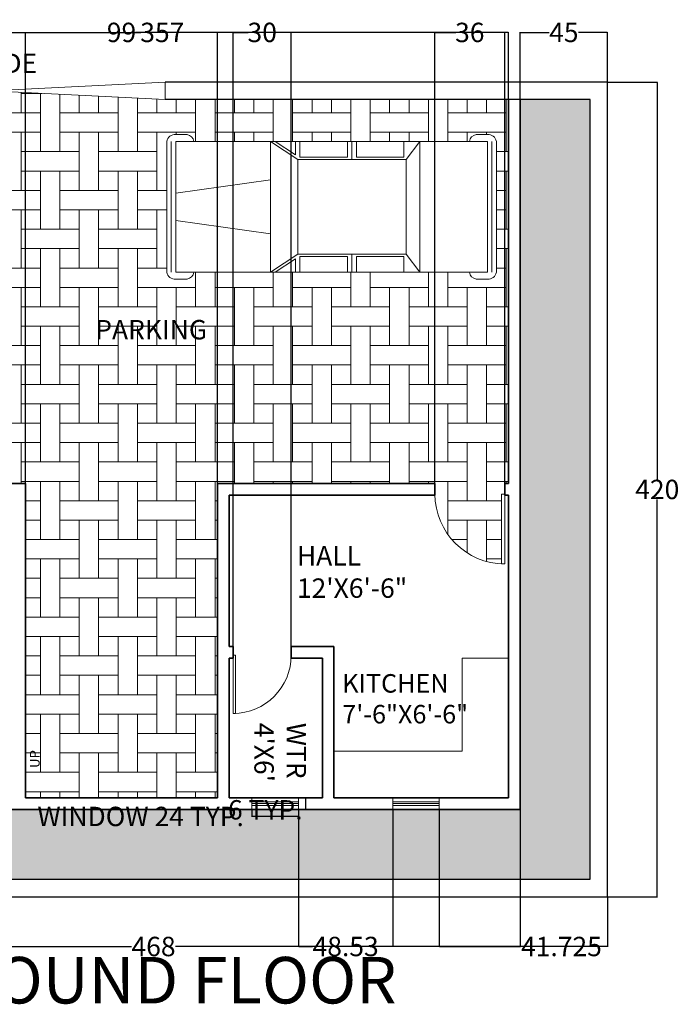
# Model space of a CAD drawing. Units: inches. Extents: x 377 to 1481, y 110 to 618.
# Tile 1 of 3: x 579 to 919, y 110 to 618. Entities that reach past the tile are written whole.
import ezdxf

# ---------------------------------------------------------------- set-up
doc = ezdxf.new("R2010")
doc.units = ezdxf.units.IN
doc.header["$MEASUREMENT"] = 0
for name, color, linetype, lineweight in [('A-ANNO-DIMS', 2, 'Continuous', 18), ('A-ANNO-TEXT', 7, 'Continuous', 18), ('A-ANNO-TITL', 7, 'Continuous', 35), ('A-AREA-IDEN', 7, 'Continuous', 18), ('A-DOOR', 4, 'Continuous', 18), ('A-EQPM-VEHI', 8, 'Continuous', 13), ('A-FLOR-FIXT', 8, 'Continuous', 20), ('A-GLAZ', 4, 'Continuous', 18), ('A-WALL', 7, 'Continuous', 35), ('C-PROP', 7, 'Continuous', 25), ('L-SITE-GATE', 3, 'Continuous', 18)]:
    doc.layers.add(name, color=color, linetype=linetype, lineweight=lineweight)
doc.layers.add('A-FLOR-PATT', color=252, linetype='Continuous', lineweight=13, true_color=0x939598)
doc.layers.add('L-PLNT-PATT', color=85, linetype='Continuous', lineweight=13, true_color=0x58ba48)
doc.styles.get("Standard").update_dxf_attribs({"font": 'arial.ttf'})
doc.dimstyles.get("Standard").update_dxf_attribs({"dimtxt": 10, "dimasz": 0.18, "dimexe": 0.18, "dimexo": 0.0625, "dimgap": 0.09, "dimtad": 0, "dimtih": 1, "dimtoh": 1, "dimdec": 0, "dimzin": 0, "dimdsep": 46, "dimlunit": 3, "dimtxsty": 'Standard', "dimcen": 0.09, "dimadec": 0, "dimazin": 0, "dimtfac": 1, "dimtdec": 0, "dimtofl": 0, "dimtmove": 0, "dimatfit": 3, "dimfxl": 1, "dimtolj": 1, "dimtzin": 0, "dimarcsym": 0})

# ---------------------------------------------------------------- blocks, each defined once
blk = doc.blocks.new('*U9')
for p, q in [((0, 0), (0, -5.999999999999999)), ((40, -6e-16), (40, -6))]:
    blk.add_line(p, q)
blk.add_lwpolyline([(0, 0), (7.1e-15, 40), (1.750000000000007, 40), (1.75, -7e-16)], close=True)
blk.add_arc((0, 0), 40, 7e-15, 90)
blk = doc.blocks.new('*U3')
for p, q in [((0, 0), (0, -5.999999999999999)), ((-40, -6e-16), (-40, -6))]:
    blk.add_line(p, q)
blk.add_lwpolyline([(0, 0), (-7.1e-15, 40), (-1.750000000000007, 40), (-1.75, -7e-16)], close=True)
blk.add_arc((0, 0), 40, 90, 180)
blk = doc.blocks.new('*U12')
for p, q in [((5.442702667415691, 42.31050314550827), (12.1182799520597, 42.31050314550827)), ((189.6886357235905, 42.31050314550827), (183.0130584389465, 42.31050314550827)), ((0.1022408397004799, -0.4060708604432933), (0.1022408397004799, 38.34966062328632)), ((2.772471753558085, -0.4131914762133988), (2.772471753558085, 38.30515677472187)), ((5.442702667415691, -0.4060708604432933), (5.442702667415691, 38.24285138673173)), ((5.446262975300346, 38.30515677472187), (16.12362632284611, 38.30515677472187)), ((16.12362632284611, 38.30515677472187), (180.3428275250889, 38.30515677472187)), ((61.5175518584254, -0.4131914762133988), (61.5175518584254, 38.30515677472187)), ((61.5175518584254, 38.30515677472187), (77.53893734157104, 27.62423311929143)), ((64.18778277228301, 38.30515677472187), (76.20382188464222, 30.29446403314904)), ((76.20382188464222, 30.29446403314904), (76.20382188464222, 38.30515677472187)), ((78.87405279849985, 38.30515677472187), (78.87405279849985, 28.95934857622023)), ((106.9114773940047, 28.95934857622023), (106.9114773940047, 38.30515677472187)), ((109.5817083078623, 27.62423311929143), (109.5817083078623, 38.30515677472187)), ((112.2519392217199, 38.30515677472187), (112.2519392217199, 28.95934857622023)), ((140.2893638172247, 28.95934857622023), (140.2893638172247, 38.30515677472187)), ((141.6244792741536, 27.62423311929143), (149.6351720157264, 38.30515677472187)), ((149.6351720157264, -0.4131914762133988), (149.6351720157264, 38.30515677472187)), ((189.685075415705, 38.30515677472187), (179.00771206816, 38.30515677472187)), ((189.6886357235905, -0.4060708604432933), (189.6886357235905, 38.24285138673173)), ((192.3588666374481, -0.4131914762133988), (192.3588666374481, 38.30515677472187)), ((195.0290975513057, -0.4060708604432933), (195.0290975513057, 38.34966062328632)), ((77.53893734157104, 27.62423311929143), (141.6244792741536, 27.62423311929143)), ((77.53893734157104, -0.4131914762133988), (77.53893734157104, 27.62423311929143)), ((78.87405279849985, 28.95934857622023), (106.9114773940047, 28.95934857622023)), ((112.2519392217199, 28.95934857622023), (140.2893638172247, 28.95934857622023)), ((141.6244792741536, -0.4131914762133988), (141.6244792741536, 27.62423311929143)), ((5.442702667415691, 7.597501265359397), (61.5175518584254, 15.60819400693222)), ((0.1022408397004799, -0.4203120919839308), (0.1022408397004799, -39.17604357571315)), ((2.772471753558085, -0.4131914762133988), (2.772471753558085, -39.13153972714869)), ((5.442702667415691, -0.4203120919839308), (5.442702667415691, -39.06923433915853)), ((61.5175518584254, -0.4131914762133988), (61.5175518584254, -39.13153972714869)), ((77.53893734157104, -0.4131914762133988), (77.53893734157104, -28.45061607171829)), ((141.6244792741536, -0.4131914762133988), (141.6244792741536, -28.45061607171829)), ((149.6351720157264, -0.4131914762133988), (149.6351720157264, -39.13153972714869)), ((189.6886357235905, -0.4203120919839308), (189.6886357235905, -39.06923433915853)), ((192.3588666374481, -0.4131914762133988), (192.3588666374481, -39.13153972714869)), ((195.0290975513057, -0.4203120919839308), (195.0290975513057, -39.17604357571315)), ((5.442702667415691, -8.423884217786224), (61.5175518584254, -16.43457695935905)), ((61.5175518584254, -39.13153972714869), (77.53893734157104, -28.45061607171829)), ((77.53893734157104, -28.45061607171829), (141.6244792741536, -28.45061607171829)), ((109.5817083078623, -28.45061607171829), (109.5817083078623, -39.13153972714869)), ((141.6244792741536, -28.45061607171829), (149.6351720157264, -39.13153972714869)), ((64.18778277228301, -39.13153972714869), (76.20382188464222, -31.12084698557587)), ((76.20382188464222, -31.12084698557587), (76.20382188464222, -39.13153972714869)), ((78.87405279849985, -39.13153972714869), (78.87405279849985, -29.78573152864706)), ((78.87405279849985, -29.78573152864706), (106.9114773940047, -29.78573152864706)), ((106.9114773940047, -29.78573152864706), (106.9114773940047, -39.13153972714869)), ((112.2519392217199, -29.78573152864706), (140.2893638172247, -29.78573152864706)), ((112.2519392217199, -39.13153972714869), (112.2519392217199, -29.78573152864706)), ((140.2893638172247, -29.78573152864706), (140.2893638172247, -39.13153972714869)), ((5.446262975300346, -39.13153972714869), (16.12362632284611, -39.13153972714869)), ((16.12362632284611, -39.13153972714869), (180.3428275250889, -39.13153972714869)), ((189.685075415705, -39.13153972714869), (179.00771206816, -39.13153972714869)), ((5.442702667415691, -43.1368860979351), (12.1182799520597, -43.1368860979351)), ((189.6886357235905, -43.1368860979351), (183.0130584389465, -43.1368860979351))]:
    blk.add_line(p, q)
for centre, radius, start, end in [((5.058189415819978, 37.26020641043229), 5.064858394326255, 85.64553999999978, 168.0943000000001), ((11.4507222235953, 37.63759904625749), 4.720341641512461, 8.130111000000149, 81.8699600000003), ((183.6806161674108, 37.63759904625749), 4.720341641512461, 98.1300399999997, 171.8698999999996), ((190.0731489751854, 37.26020641043229), 5.064858394326255, 11.90573999999997, 94.35446000000022), ((5.058189415819978, -38.08658936285912), 5.064858394326255, 191.9056999999999, 274.3545000000004), ((11.4507222235953, -38.46398199868429), 4.720341641512461, 278.1300000000006, 351.8698999999996), ((183.6806161674108, -38.46398199868429), 4.720341641512461, 188.1301000000004, 261.8699999999993), ((190.0731489751854, -38.08658936285912), 5.064858394326255, 265.6454999999995, 348.0943000000001)]:
    blk.add_arc(centre, radius, start, end)
blk = doc.blocks.new('WIN-24IN')
for p, q in [((8.90267408522e-05, 6.000397743999627), (8.90267408522e-05, 0.0003977439995708)), ((24.00008902674085, 6.000397743999627), (24.00008902674085, 0.0003977439995708)), ((24.00008902674085, 4.000397743999599), (8.90267408522e-05, 4.000397743999599)), ((24.00008902674085, 3.000397743999599), (8.90267408522e-05, 3.000397743999599)), ((24.00008902674085, 2.000397743999599), (8.90267408522e-05, 2.000397743999599))]:
    blk.add_line(p, q)
blk = doc.blocks.new('*D17')
at = {"layer": 'A-ANNO-DIMS', "color": 0, "lineweight": -2, "transparency": 16777216}
for p, q in [((699.0626046596035, 210.7768977439996), (699.0626046596035, 207.0593977439996)), ((723.0626046596035, 210.7768977439996), (723.0626046596035, 207.0593977439996)), ((699.0626046596035, 207.2393977439996), (698.8826046596034, 207.2393977439996)), ((722.8826046596035, 207.2393977439996), (699.2426046596034, 207.2393977439996))]:
    blk.add_line(p, q, dxfattribs=at)
at = {"layer": 'A-ANNO-DIMS', "color": 0, "lineweight": 100, "transparency": 16777216}
for points in [[(699.2426046596034, 207.2693977439996), (699.2426046596034, 207.2093977439996), (699.0626046596035, 207.2393977439996)], [(722.8826046596035, 207.2693977439996), (722.8826046596035, 207.2093977439996), (723.0626046596035, 207.2393977439996)]]:
    blk.add_solid(points, dxfattribs=at)
at = {"layer": 'Defpoints', "color": 0, "lineweight": 100, "transparency": 16777216}
for p in [(699.0626046596035, 210.8393977439996), (723.0626046596035, 210.8393977439996), (699.0626046596035, 207.2393977439996)]:
    blk.add_point(p, dxfattribs=at)
at = {"layer": 'A-ANNO-DIMS', "color": 0, "transparency": 16777216, "insert": (641.6609539092624, 207.2393977439996), "char_height": 10, "attachment_point": 5}
blk.add_mtext('\\A1;WINDOW 24 TYP.', dxfattribs=at)
blk = doc.blocks.new('*D18')
at = {"layer": 'A-ANNO-DIMS', "color": 0, "lineweight": -2, "transparency": 16777216}
for p, q in [((723.1251046596037, 216.8393977439997), (726.8426046596039, 216.8393977439997)), ((726.6626046596039, 216.6593977439998), (726.6626046596039, 211.0193977439997)), ((723.1251046596037, 210.8393977439997), (726.8426046596039, 210.8393977439997)), ((726.6626046596039, 210.6593977439997), (726.482604659604, 210.6593977439997)), ((726.6626046596039, 210.8393977439997), (726.6626046596039, 210.6593977439997))]:
    blk.add_line(p, q, dxfattribs=at)
at = {"layer": 'A-ANNO-DIMS', "color": 0, "lineweight": 100, "transparency": 16777216}
for points in [[(726.632604659604, 216.6593977439998), (726.692604659604, 216.6593977439998), (726.6626046596039, 216.8393977439997)], [(726.632604659604, 211.0193977439997), (726.692604659604, 211.0193977439997), (726.6626046596039, 210.8393977439997)]]:
    blk.add_solid(points, dxfattribs=at)
at = {"layer": 'Defpoints', "color": 0, "lineweight": 100, "transparency": 16777216}
for p in [(723.0626046596037, 216.8393977439997), (723.0626046596037, 210.8393977439997), (726.6626046596039, 210.8393977439997)]:
    blk.add_point(p, dxfattribs=at)
at = {"layer": 'A-ANNO-DIMS', "color": 0, "transparency": 16777216, "insert": (705.9117042503268, 210.6593977439994), "char_height": 10, "attachment_point": 5}
blk.add_mtext('\\A1;6 TYP.', dxfattribs=at)
blk = doc.blocks.new('*D27')
at = {"layer": 'A-ANNO-DIMS', "color": 0, "lineweight": -2, "transparency": 16777216}
for p, q in [((414.320847, 165.776898), (414.320847, 140.009398)), ((882.3208469999998, 165.776898), (882.3208469999998, 140.009398)), ((414.500847, 140.189398), (636.9723203969986, 140.189398)), ((882.1408469999999, 140.189398), (659.6693736030013, 140.189398))]:
    blk.add_line(p, q, dxfattribs=at)
at = {"layer": 'A-ANNO-DIMS', "color": 0, "lineweight": 100, "transparency": 16777216}
for points in [[(414.500847, 140.219398), (414.500847, 140.159398), (414.320847, 140.189398)], [(882.1408469999999, 140.219398), (882.1408469999999, 140.159398), (882.3208469999998, 140.189398)]]:
    blk.add_solid(points, dxfattribs=at)
at = {"layer": 'Defpoints', "color": 0, "lineweight": 100, "transparency": 16777216}
for p in [(414.320847, 165.839398), (882.3208469999998, 165.839398), (882.3208469999998, 140.189398)]:
    blk.add_point(p, dxfattribs=at)
at = {"layer": 'A-ANNO-DIMS', "color": 0, "transparency": 16777216, "insert": (648.320847, 140.189398), "char_height": 10, "attachment_point": 5}
blk.add_mtext('\\A1;468', dxfattribs=at)
blk = doc.blocks.new('*D28')
at = {"layer": 'A-ANNO-DIMS', "color": 0, "lineweight": -2, "transparency": 16777216}
for p, q in [((882.3833470000003, 585.8393980000001), (908.1508470000009, 585.8393980000001)), ((907.970847000001, 585.6593980000002), (907.970847000001, 381.035127877217)), ((907.970847000001, 166.019398), (907.970847000001, 370.6436681227832)), ((882.3833470000003, 165.839398), (908.1508470000009, 165.839398))]:
    blk.add_line(p, q, dxfattribs=at)
at = {"layer": 'A-ANNO-DIMS', "color": 0, "lineweight": 100, "transparency": 16777216}
for points in [[(907.9408470000009, 585.6593980000002), (908.0008470000009, 585.6593980000002), (907.970847000001, 585.8393980000001)], [(907.9408470000011, 166.019398), (908.0008470000009, 166.019398), (907.970847000001, 165.839398)]]:
    blk.add_solid(points, dxfattribs=at)
at = {"layer": 'Defpoints', "color": 0, "lineweight": 100, "transparency": 16777216}
for p in [(882.3208470000004, 585.8393980000001), (907.970847000001, 585.8393980000001), (882.3208470000004, 165.839398)]:
    blk.add_point(p, dxfattribs=at)
at = {"layer": 'A-ANNO-DIMS', "color": 0, "transparency": 16777216, "insert": (907.9708470000008, 375.8393979999998), "char_height": 10, "attachment_point": 5}
blk.add_mtext('\\A1;420', dxfattribs=at)
blk = doc.blocks.new('*D30')
at = {"layer": 'A-ANNO-DIMS', "color": 0, "lineweight": -2, "transparency": 16777216}
for p, q in [((474.31833, 576.9018979999998), (474.31833, 611.6693979999999)), ((474.49833, 611.489398), (641.6859322926329, 611.489398)), ((831.1408469999999, 611.489398), (663.953244707367, 611.489398)), ((831.3208469999998, 576.9018979999998), (831.3208469999998, 611.6693979999999))]:
    blk.add_line(p, q, dxfattribs=at)
at = {"layer": 'A-ANNO-DIMS', "color": 0, "lineweight": 100, "transparency": 16777216}
for points in [[(474.49833, 611.519398), (474.49833, 611.4593980000001), (474.31833, 611.489398)], [(831.1408469999999, 611.519398), (831.1408469999999, 611.4593980000001), (831.3208469999998, 611.489398)]]:
    blk.add_solid(points, dxfattribs=at)
at = {"layer": 'Defpoints', "color": 0, "lineweight": 100, "transparency": 16777216}
for p in [(831.3208469999998, 611.489398), (474.31833, 576.8393979999998), (831.3208469999998, 576.8393979999998)]:
    blk.add_point(p, dxfattribs=at)
at = {"layer": 'A-ANNO-DIMS', "color": 0, "transparency": 16777216, "insert": (652.8195885, 611.489398), "char_height": 10, "attachment_point": 5}
blk.add_mtext('\\A1;357', dxfattribs=at)
blk = doc.blocks.new('*D31')
at = {"layer": 'A-ANNO-DIMS', "color": 0, "lineweight": -2, "transparency": 16777216}
for p, q in [((837.3208469999998, 576.9018979999998), (837.3208469999998, 611.6693979999999)), ((837.5008469999999, 611.489398), (852.3297555948158, 611.489398)), ((882.1408469999999, 611.489398), (867.3119384051842, 611.489398)), ((882.3208469999998, 585.901898), (882.3208469999998, 611.6693979999999))]:
    blk.add_line(p, q, dxfattribs=at)
at = {"layer": 'A-ANNO-DIMS', "color": 0, "lineweight": 100, "transparency": 16777216}
for points in [[(837.5008469999999, 611.519398), (837.5008469999999, 611.4593980000001), (837.3208469999998, 611.489398)], [(882.1408469999999, 611.519398), (882.1408469999999, 611.4593980000001), (882.3208469999998, 611.489398)]]:
    blk.add_solid(points, dxfattribs=at)
at = {"layer": 'Defpoints', "color": 0, "lineweight": 100, "transparency": 16777216}
for p in [(882.3208469999998, 611.489398), (882.3208469999998, 585.8393979999998), (837.3208469999998, 576.8393979999998)]:
    blk.add_point(p, dxfattribs=at)
at = {"layer": 'A-ANNO-DIMS', "color": 0, "transparency": 16777216, "insert": (859.8208469999998, 611.489398), "char_height": 10, "attachment_point": 5}
blk.add_mtext('\\A1;45', dxfattribs=at)
blk = doc.blocks.new('*D35')
at = {"layer": 'A-ANNO-DIMS', "color": 0, "lineweight": -2, "transparency": 16777216}
for p, q in [((582.31833, 216.901898), (582.31833, 611.669398)), ((582.4983299999998, 611.489398), (624.5570100552522, 611.489398)), ((681.1408469999999, 611.489398), (639.0821669447477, 611.489398)), ((681.3208469999998, 216.901898), (681.3208469999998, 611.669398))]:
    blk.add_line(p, q, dxfattribs=at)
at = {"layer": 'A-ANNO-DIMS', "color": 0, "lineweight": 100, "transparency": 16777216}
for points in [[(582.4983299999998, 611.519398), (582.4983299999998, 611.4593980000001), (582.31833, 611.489398)], [(681.1408469999999, 611.519398), (681.1408469999999, 611.4593980000001), (681.3208469999998, 611.489398)]]:
    blk.add_solid(points, dxfattribs=at)
at = {"layer": 'Defpoints', "color": 0, "lineweight": 100, "transparency": 16777216}
for p in [(681.3208469999998, 611.489398), (582.31833, 216.839398), (681.3208469999998, 216.839398)]:
    blk.add_point(p, dxfattribs=at)
at = {"layer": 'A-ANNO-DIMS', "color": 0, "transparency": 16777216, "insert": (631.8195885, 611.489398), "char_height": 10, "attachment_point": 5}
blk.add_mtext('\\A1;99', dxfattribs=at)
blk = doc.blocks.new('*D36')
at = {"layer": 'A-ANNO-DIMS', "color": 0, "lineweight": -2, "transparency": 16777216}
for p, q in [((793.3208469999998, 378.901898), (793.3208469999998, 611.6693979999999)), ((793.5008469999999, 611.489398), (804.075321761255, 611.489398)), ((829.140847, 611.489398), (818.5663722387449, 611.489398)), ((829.3208469999998, 378.901898), (829.3208469999998, 611.6693979999999))]:
    blk.add_line(p, q, dxfattribs=at)
at = {"layer": 'A-ANNO-DIMS', "color": 0, "lineweight": 100, "transparency": 16777216}
for points in [[(793.5008469999999, 611.519398), (793.5008469999999, 611.4593980000001), (793.3208469999998, 611.489398)], [(829.140847, 611.519398), (829.140847, 611.4593980000001), (829.3208469999998, 611.489398)]]:
    blk.add_solid(points, dxfattribs=at)
at = {"layer": 'Defpoints', "color": 0, "lineweight": 100, "transparency": 16777216}
for p in [(829.3208469999998, 611.489398), (793.3208469999998, 378.839398), (829.3208469999998, 378.839398)]:
    blk.add_point(p, dxfattribs=at)
at = {"layer": 'A-ANNO-DIMS', "color": 0, "transparency": 16777216, "insert": (811.320847, 611.489398), "char_height": 10, "attachment_point": 5}
blk.add_mtext('\\A1;36', dxfattribs=at)
blk = doc.blocks.new('*D37')
at = {"layer": 'A-ANNO-DIMS', "color": 0, "lineweight": -2, "transparency": 16777216}
for p, q in [((689.3208469999998, 294.901898), (689.3208469999998, 611.6693979999999)), ((689.5008469999999, 611.489398), (697.0889643260573, 611.489398)), ((719.1408469999999, 611.489398), (711.5527296739426, 611.489398)), ((719.320847, 294.901898), (719.320847, 611.6693979999999))]:
    blk.add_line(p, q, dxfattribs=at)
at = {"layer": 'A-ANNO-DIMS', "color": 0, "lineweight": 100, "transparency": 16777216}
for points in [[(689.5008469999999, 611.519398), (689.5008469999999, 611.4593980000001), (689.3208469999998, 611.489398)], [(719.1408469999999, 611.519398), (719.1408469999999, 611.4593980000001), (719.320847, 611.489398)]]:
    blk.add_solid(points, dxfattribs=at)
at = {"layer": 'Defpoints', "color": 0, "lineweight": 100, "transparency": 16777216}
for p in [(719.320847, 611.489398), (689.3208469999998, 294.839398), (719.320847, 294.839398)]:
    blk.add_point(p, dxfattribs=at)
at = {"layer": 'A-ANNO-DIMS', "color": 0, "transparency": 16777216, "insert": (704.3208469999998, 611.489398), "char_height": 10, "attachment_point": 5}
blk.add_mtext('\\A1;30', dxfattribs=at)
blk = doc.blocks.new('*D38')
at = {"layer": 'A-ANNO-DIMS', "color": 0, "lineweight": -2, "transparency": 16777216}
for p, q in [((723.0626049999998, 210.776898), (723.0626049999998, 140.009398)), ((771.596188, 210.776898), (771.596188, 140.009398)), ((723.2426049999999, 140.189398), (730.1657266500682, 140.189398)), ((771.416188, 140.189398), (764.4930663499318, 140.189398))]:
    blk.add_line(p, q, dxfattribs=at)
at = {"layer": 'A-ANNO-DIMS', "color": 0, "lineweight": 100, "transparency": 16777216}
for points in [[(723.2426049999999, 140.219398), (723.2426049999999, 140.159398), (723.0626049999998, 140.189398)], [(771.416188, 140.219398), (771.416188, 140.159398), (771.596188, 140.189398)]]:
    blk.add_solid(points, dxfattribs=at)
at = {"layer": 'Defpoints', "color": 0, "lineweight": 100, "transparency": 16777216}
for p in [(723.0626049999998, 210.839398), (771.596188, 210.839398), (771.596188, 140.189398)]:
    blk.add_point(p, dxfattribs=at)
at = {"layer": 'A-ANNO-DIMS', "color": 0, "transparency": 16777216, "insert": (747.3293965, 140.189398), "char_height": 10, "attachment_point": 5}
blk.add_mtext('\\A1;48.53', dxfattribs=at)
blk = doc.blocks.new('*D39')
at = {"layer": 'A-ANNO-DIMS', "color": 0, "lineweight": -2, "transparency": 16777216}
for p, q in [((795.596188, 210.776898), (795.596188, 140.009398)), ((837.3208469999998, 210.776898), (837.3208469999998, 140.009398)), ((795.7761879999999, 140.189398), (837.140847, 140.189398)), ((837.3208469999998, 140.189398), (837.500847, 140.189398))]:
    blk.add_line(p, q, dxfattribs=at)
at = {"layer": 'A-ANNO-DIMS', "color": 0, "lineweight": 100, "transparency": 16777216}
for points in [[(795.7761879999999, 140.219398), (795.7761879999999, 140.159398), (795.596188, 140.189398)], [(837.140847, 140.219398), (837.140847, 140.159398), (837.3208469999998, 140.189398)]]:
    blk.add_solid(points, dxfattribs=at)
at = {"layer": 'Defpoints', "color": 0, "lineweight": 100, "transparency": 16777216}
for p in [(795.596188, 210.839398), (837.3208469999998, 210.839398), (837.3208469999998, 140.189398)]:
    blk.add_point(p, dxfattribs=at)
at = {"layer": 'A-ANNO-DIMS', "color": 0, "transparency": 16777216, "insert": (858.5867542305592, 140.189398), "char_height": 10, "attachment_point": 5}
blk.add_mtext('\\A1;41.725', dxfattribs=at)

msp = doc.modelspace()

# ---------------------------------------------------------------- hatches: boundary and pattern name
at = {"layer": 'A-FLOR-PATT'}
h = msp.add_hatch(dxfattribs=at)
h.set_pattern_fill('±ÀÖ¯²ÄÁÏ', color=256, scale=20)
h.set_pattern_definition([(0, (0, 0), (20, 20), [30, -10]), (0, (0, 10), (20, 20), [30, -10]), (90, (10, 10), (-20, 20), [30, -10]), (90, (20, 10), (-20, 20), [30, -10])])
h.paths.add_polyline_path([(831.3208470620848, 576.8393977439996), (654.3183302215624, 576.8393977439996), (564.3183302215629, 581.3393977439996), (474.3183302215626, 576.8393977439996), (474.3183302215626, 378.8393977439996), (582.3183302215626, 378.8393977439995), (582.3183302215626, 216.8393977439996), (681.320847062085, 216.8393977439997), (681.3208470620849, 378.8393977439995), (793.3762999136519, 378.8393977439995), (793.3762999136519, 373.4477156717346, 0.4014527144963569), (827.7482731243409, 337.537585054926), (827.7482731243409, 373.4477156717346), (829.3208470620848, 373.4477156717346), (829.3208470620848, 378.8393977439996), (831.3208470620848, 378.8393977439995)])
h.paths.add_polyline_path([(655.1112320992189, 487.8017993641329), (655.1112320992189, 521.5563777088427), (655.1112320992189, 555.3233738998766, -0.3760864404517753), (659.767292319398, 558.8161256031975), (665.5887632688018, 558.8161256031975, -0.3333350785240507), (669.0813054040638, 555.3236063246482), (669.0813092134161, 555.3236063246482), (811.1104303504404, 555.3236063246482, -0.3333350785240531), (814.6029724857026, 558.8161256031975), (820.4244434351054, 558.8161256031975, -0.3760864404519927), (825.0805036552854, 555.3233738998733), (825.0805036552854, 521.5687955551666), (825.0805036552854, 487.8017993641362, -0.3760864404520696), (820.4244434351043, 484.3090476608121), (814.6029724857024, 484.3090476608121, -0.3333350785240366), (811.1104303504404, 487.8015669393615), (811.1104265410881, 487.8015669393615), (669.0813054040638, 487.8015669393615, -0.3333350785240358), (665.588763268802, 484.3090476608121), (659.7672923193994, 484.3090476608121, -0.3760864404518541)], flags=16)
h.paths.add_polyline_path([(659.7679244706181, 521.5563777088427), (659.7679244706181, 528.5476251891034), (708.6631943703085, 535.532663746202), (708.6631943703085, 555.3236063246482), (722.6332714845057, 546.01022158185), (778.5135799412946, 546.01022158185), (785.4986184983933, 555.3236063246482), (785.4986184983933, 521.5625866320047), (785.4986184983933, 487.8015669393614), (778.5135799412946, 497.1149516821596), (722.6332714845057, 497.1149516821596), (708.6631943703085, 487.8015669393615), (708.6631943703085, 507.5925095178076), (659.7679244706181, 514.5775480749062)], flags=0)
edge = h.paths.add_edge_path(flags=16)
edge.add_ellipse((512.141418614859, 584.5696558424829), major_axis=(-204.7255748268525, 9.67931e-11), ratio=0.8423038695443797, start_angle=100.2095389971704, end_angle=102.44462729347111, ccw=False)
edge.add_ellipse((565.7338664611478, 273.648778987746), major_axis=(168.2852536317261, 6.42065e-11), ratio=0.842303869543657, start_angle=99.25656600717964, end_angle=102.5549326441154)
edge.add_line((534.707768362197, 412.9662154153117), (530.5983486771285, 410.6938254662535))
edge.add_line((530.5983486771285, 410.6938254662535), (526.4889289920602, 412.9662154153116))
edge.add_ellipse((495.4628308931093, 273.648778987746), major_axis=(168.2852536315943, 6.1815e-11), ratio=0.8423038695442986, start_angle=77.44506735584166, end_angle=80.74343399277738)
edge.add_ellipse((549.0552787394023, 584.5696558424856), major_axis=(204.7255748269201, 3.28788e-11), ratio=0.8423038695441253, start_angle=257.5553727065455, end_angle=259.7904610028463, ccw=False)
edge.add_ellipse((928.8888750783977, 435.9044437085582), major_axis=(-417.9823698359099, 1.184e-13), ratio=0.842303869543927, start_angle=-2.1985405659551134, end_angle=2.8637146078376077, ccw=False)
edge.add_ellipse((526.9857163546047, 500.9000910277084), major_axis=(60.20166025916774, 4.181e-13), ratio=0.8423038695439812, start_angle=252.2800467772492, end_angle=265.917589308849)
edge.add_line((523.3730840320812, 450.283383470902), (537.8236133221772, 450.283383470902))
edge.add_ellipse((534.2109809996527, 500.9000910277083), major_axis=(60.201660259169, 1.2736e-12), ratio=0.8423038695439622, start_angle=-85.91758930885108, end_angle=-72.28004677725126)
edge.add_ellipse((132.3078222758608, 435.9044437085587), major_axis=(-417.9823698359087, 2.3459e-12), ratio=0.8423038695438743, start_angle=177.1362853921626, end_angle=182.1985405659555, ccw=False)
edge = h.paths.add_edge_path(flags=16)
edge.add_ellipse((534.2109809996541, 501.4974298966528), major_axis=(54.83387102201502, 2.4993e-12), ratio=0.8423038695439453, start_angle=-85.7225790369485, end_angle=-68.16504620329431, ccw=False)
edge.add_line((537.6586440135299, 455.4020319851987), (523.5380533407272, 455.4020319851987))
edge.add_ellipse((526.985716354604, 501.4974298966517), major_axis=(-54.8338710220135, 2.0245e-12), ratio=0.8423038695439498, start_angle=68.16504620329238, end_angle=85.72257903694663, ccw=False)
edge.add_line((509.4513084570433, 457.7357275014352), (510.9164148538646, 468.7168197280619))
edge.add_ellipse((528.721139195539, 511.0893217744386), major_axis=(53.3633742937202, 3.469e-13), ratio=0.8423038695439728, start_angle=247.2080851224096, end_angle=265.1299304028639)
edge.add_line((524.9011977337861, 466.2564549519428), (536.295499620471, 466.2564549519428))
edge.add_ellipse((532.4755581587168, 511.0893217744494), major_axis=(53.36337429373605, 3.8424e-12), ratio=0.8423038695439261, start_angle=-85.12993040286842, end_angle=-67.20808512241756)
edge.add_line((550.2802825003928, 468.7168197280617), (551.7453888972141, 457.735727501435))
edge = h.paths.add_edge_path(flags=0)
edge.add_line((542.111699473761, 444.9337137407289), (542.111699473761, 435.0025221262431))
edge.add_line((542.111699473761, 435.0025221262431), (538.2562464159993, 432.3163569622979))
edge.add_line((538.2562464159993, 432.3163569622979), (536.972632243019, 432.3163569622979))
edge.add_line((536.972632243019, 432.3163569622979), (536.972632243019, 430.7404435434111))
edge.add_ellipse((499.3077352576486, 430.740443543411), major_axis=(-37.66489698537048, 7.634e-13), ratio=0.8423038695439682, start_angle=150.5614304020218, end_angle=180.0000000000012, ccw=False)
edge.add_ellipse((561.8889620966085, 430.740443543411), major_axis=(37.66489698537043, 6.965e-13), ratio=0.8423038695439699, start_angle=179.9999999999989, end_angle=209.4385695979783, ccw=False)
edge.add_line((524.2240651112381, 430.7404435434107), (524.2240651112381, 432.3163569622979))
edge.add_line((524.2240651112381, 432.3163569622979), (522.940450938258, 432.3163569622979))
edge.add_line((522.940450938258, 432.3163569622979), (519.0849978804961, 435.0025221262431))
edge.add_line((519.0849978804961, 435.0025221262431), (519.0849978804961, 444.9337137407288))
edge.add_ellipse((521.6545314958671, 444.8340445689326), major_axis=(0.2391293983204887, 4.251437037044111), ratio=0.6038335755719065, start_angle=-73.65740804569998, end_angle=90.99798572497588, ccw=False)
edge.add_line((524.2240651112381, 445.4330946490179), (524.2240651112381, 430.7404435434109))
edge.add_ellipse((561.8889620966085, 430.740443543411), major_axis=(37.66489698537043, 6.965e-13), ratio=0.8423038695439699, start_angle=179.9999999999989, end_angle=209.4385695979783)
edge.add_ellipse((499.3077352576486, 430.740443543411), major_axis=(-37.66489698537048, 7.634e-13), ratio=0.8423038695439682, start_angle=150.5614304020218, end_angle=180.0000000000011)
edge.add_line((536.972632243019, 430.7404435434112), (536.972632243019, 445.4330946490189))
edge.add_ellipse((539.5421658583901, 444.8340445689326), major_axis=(-0.2391293983215679, 4.251437037044156), ratio=0.6038335755718898, start_angle=269.00201427500974, end_angle=433.6574080456862, ccw=False)
edge = h.paths.add_edge_path(flags=16)
edge.add_ellipse((530.5983486771285, 422.2304898077624), major_axis=(-98.58514223035905, 4.876e-13), ratio=0.8423038695439689, start_angle=256.4018653097696, end_angle=283.5981346902308)
edge.add_line((510.9164148538645, 503.5974436099374), (510.9164148538645, 516.2199560207953))
edge.add_ellipse((530.5983486771285, 434.8530022186204), major_axis=(98.5851422303597, 9.36e-14), ratio=0.8423038695439631, start_angle=76.40186530976939, end_angle=103.5981346902305, ccw=False)
edge.add_line((550.2802825003926, 516.2199560207953), (550.2802825003928, 503.5974436099373))
edge = h.paths.add_edge_path(flags=16)
edge.add_ellipse((548.2956151630524, 522.7658727769762), major_axis=(1.98466733734017, 1.09e-13), ratio=0.8423038695439435, start_angle=269.9999999999969, end_angle=359.9999999999969, ccw=False)
edge.add_line((548.2956151630524, 521.094179798977), (512.9010821912045, 521.0941797989772))
edge.add_ellipse((512.9010821912045, 522.7658727769762), major_axis=(1.984667337340112, 5.52e-14), ratio=0.8423038695439679, start_angle=179.9999999999985, end_angle=269.9999999999984, ccw=False)
edge.add_line((510.9164148538645, 522.7658727769762), (510.9164148538645, 535.8181149898111))
edge.add_line((510.9164148538645, 535.8181149898111), (550.2802825003924, 535.8181149898103))
edge.add_line((550.2802825003924, 535.8181149898103), (550.2802825003926, 522.7658727769762))
h.paths.add_polyline_path([(592.3367361683343, 230.4436529032155), (592.3367361683343, 242.646927118768), (582.0331891014856, 242.646927118768), (582.0331891014856, 230.4436529032155)], flags=24)
at = {"layer": 'L-PLNT-PATT'}
h = msp.add_hatch(color=256, dxfattribs=at)
h.dxf.hatch_style = 1
h.paths.add_polyline_path([(468.3183302215627, 576.8393977439996), (446.8212432498917, 576.8393977439996), (423.8498146784631, 174.8393977439996), (873.320847062085, 174.8393977439996), (873.3208470620846, 576.8393977439996), (837.3208470620848, 576.8393977439996), (837.3208470620848, 210.8393977439996), (467.9754730787054, 210.8393977439996), (468.3183302215626, 216.8393977440005)])

# ---------------------------------------------------------------- linework, layer by layer
at = {"layer": 'A-FLOR-FIXT'}
for p, q in [((807.3208470620848, 288.8393977439996), (831.3208470620848, 288.8393977439997)), ((807.320847062085, 240.8393977439996), (807.320847062085, 288.8393977439997)), ((741.320847062085, 240.8393977439996), (807.320847062085, 240.8393977439997))]:
    msp.add_line(p, q, dxfattribs=at)
at = {"layer": 'A-WALL'}
for p, q in [((831.3208470620848, 378.8393977439995), (831.3208470620848, 576.8393977439996)), ((837.3208470620848, 210.8393977439996), (837.3208470620848, 576.8393977439996)), ((474.3183302215626, 378.8393977439996), (582.3183302215626, 378.8393977439995)), ((582.3183302215626, 216.8393977439996), (582.3183302215626, 378.8393977439995)), ((681.320847062085, 216.8393977439996), (681.3208470620849, 378.8393977439995)), ((681.3208470620849, 378.8393977439995), (793.3208470620849, 378.8393977439995)), ((793.320847062085, 372.8393977439997), (793.3208470620849, 378.8393977439996)), ((829.3208470620848, 372.8393977439996), (829.3208470620848, 378.8393977439996)), ((829.3208470620848, 378.8393977439996), (831.3208470620848, 378.8393977439995)), ((687.320847062085, 372.8393977439996), (793.3208470620849, 372.8393977439996)), ((687.3208470620848, 294.8393977439995), (687.320847062085, 372.8393977439996)), ((831.3208470620848, 372.8393977439996), (829.3208470620848, 372.8393977439996)), ((831.3208470620848, 294.8393977439996), (831.320847062085, 372.8393977439996)), ((689.3208470620849, 294.8393977439994), (687.3208470620848, 294.8393977439995)), ((689.3208470620849, 288.8393977439994), (689.3208470620849, 294.8393977439994)), ((719.3208470620849, 294.8393977439995), (741.3208470620848, 294.8393977439995)), ((719.3208470620849, 288.8393977439995), (719.3208470620849, 294.8393977439995)), ((741.320847062085, 216.8393977439996), (741.3208470620848, 294.8393977439996)), ((831.3208470620848, 216.8393977439996), (831.3208470620848, 294.8393977439996)), ((687.3208470620848, 216.8393977439996), (687.3208470620848, 288.8393977439994)), ((687.3208470620848, 288.8393977439994), (689.3208470620849, 288.8393977439994)), ((719.3208470620849, 288.8393977439995), (735.320847062085, 288.8393977439996)), ((735.320847062085, 216.8393977439996), (735.320847062085, 288.8393977439996)), ((582.3183302215626, 216.8393977439996), (681.3208470620849, 216.8393977439996)), ((687.3208470620848, 216.8393977439996), (735.3208470620851, 216.8393977439996)), ((741.320847062085, 216.8393977439996), (831.320847062085, 216.8393977439996)), ((467.9754730787053, 210.8393977439996), (837.3208470620848, 210.8393977439996))]:
    msp.add_line(p, q, dxfattribs=at)
at = {"layer": 'C-PROP'}
for p, q in [((882.3208470620848, 585.8393977439996), (654.3183302215626, 585.8393977439996)), ((882.3208470620848, 165.8393977439996), (882.3208470620848, 585.8393977439996)), ((873.3208470620846, 576.8393977439996), (654.3183302215626, 576.8393977439996)), ((873.320847062085, 174.8393977439996), (873.3208470620846, 576.8393977439996)), ((423.8498146784632, 174.8393977439996), (873.3208470620848, 174.8393977439996)), ((414.3208470620847, 165.8393977439996), (882.3208470620848, 165.8393977439996))]:
    msp.add_line(p, q, dxfattribs=at)
at = {"layer": 'L-SITE-GATE'}
for p, q in [((654.3183302215626, 576.8393977439996), (474.3183302215626, 585.8393977439996)), ((474.3183302215626, 576.8393977439996), (654.3183302215626, 585.8393977439996)), ((654.3183302215626, 576.8393977439995), (654.3183302215626, 585.8393977439996))]:
    msp.add_line(p, q, dxfattribs=at)

# ---------------------------------------------------------------- block references
at = {"layer": 'A-DOOR', "rotation": 180}
for name, p, xscale, yscale, zscale in [('*U9', (829.3208470620848, 373.4477156717346), 0.8986136787108254, 0.8986136787108254, 0.8986136787108254), ('*U3', (689.3208470620849, 290.343693014185), 0.7492841216357637, 0.7492841216357637, 0.7492841216357637)]:
    msp.add_blockref(name, p, dxfattribs=dict(at, xscale=xscale, yscale=yscale, zscale=zscale))
at = {"layer": 'A-EQPM-VEHI', "xscale": 0.8719643584441334, "yscale": 0.8719643584441334, "zscale": 0.8719643584441334}
msp.add_blockref('*U12', (655.0220817310227, 521.9228748724757), dxfattribs=at)
at = {"layer": 'A-GLAZ', "rotation": 180}
for p in [(723.0626936863443, 216.8397954879992), (795.5962769266059, 216.8397954879992)]:
    msp.add_blockref('WIN-24IN', p, dxfattribs=at)

# ---------------------------------------------------------------- texts
at = {"layer": 'A-ANNO-TEXT', "insert": (532.9243151521782, 617.2521118760563), "char_height": 10, "attachment_point": 1}
msp.add_mtext_dynamic_manual_height_columns("GATE\\P15' WIDE", width=70.11836276200438, gutter_width=1, heights=[0], dxfattribs=at)
at = {"layer": 'A-ANNO-TEXT', "insert": (584.6065178872974, 232.2427661365034), "char_height": 5, "attachment_point": 1, "rotation": 90}
msp.add_mtext_dynamic_manual_height_columns('UP', width=12.28670037788015, gutter_width=1, heights=[0], dxfattribs=at)
at = {"layer": 'A-ANNO-TITL', "insert": (523.5625681240535, 134.8117828229256), "char_height": 24, "attachment_point": 1}
msp.add_mtext_dynamic_manual_height_columns('{\\fTimes New Roman|b0|i0|c0|p18;GROUND FLOOR}', width=313.0421048124909, gutter_width=1, heights=[94.3060019033042], dxfattribs=at)
at = {"layer": 'A-AREA-IDEN', "attachment_point": 1}
for s, width, gutter_width, insert, char_height in [('PARKING', 70.11836276200438, 1, (618.260086650378, 463.223073384904), 10), ('HALL\\P12\'X6\'-6"', 70.11836276200438, 1, (722.2031241632903, 346.633005003926), 10), ('KITCHEN\\P7\'-6"X6\'-6"', 66.7973367241912, 0.9526368570657389, (745.6010781962208, 280.6209993285462), 9.52636857065739)]:
    msp.add_mtext_dynamic_manual_height_columns(s, width=width, gutter_width=gutter_width, heights=[0], dxfattribs=dict(at, insert=insert, char_height=char_height))
at = {"layer": 'A-AREA-IDEN', "insert": (726.9712995742854, 255.5527991159774), "char_height": 10, "attachment_point": 1, "rotation": 270}
msp.add_mtext_dynamic_manual_height_columns("WTR\\P4'X6'", width=70.11836276200438, gutter_width=1, heights=[0], dxfattribs=at)

# ---------------------------------------------------------------- dimensions: what is measured, and where the dimension line sits
at = {"layer": 'A-ANNO-DIMS'}
for base, p1, p2, override, picture, middle in [((831.3208469999998, 611.489398), (474.31833, 576.8393979999998), (831.3208469999998, 576.8393979999998), {"dimdec": 0, "dimlfac": 1, "dimrnd": 0, "dimzin": 0, "dimdsep": 46, "dimlunit": 2}, '*D30', (652.8195885, 611.489398)), ((681.3208469999998, 611.489398), (582.31833, 216.839398), (681.3208469999998, 216.839398), {"dimdec": 0, "dimlfac": 1, "dimrnd": 0, "dimzin": 0, "dimdsep": 46, "dimlunit": 2}, '*D35', (631.8195885, 611.489398)), ((719.320847, 611.489398), (689.3208469999998, 294.839398), (719.320847, 294.839398), {"dimdec": 0, "dimlfac": 1, "dimrnd": 0, "dimzin": 0, "dimdsep": 46, "dimlunit": 2}, '*D37', (704.3208469999998, 611.489398)), ((829.3208469999998, 611.489398), (793.3208469999998, 378.839398), (829.3208469999998, 378.839398), {"dimdec": 0, "dimlfac": 1, "dimrnd": 0, "dimzin": 0, "dimdsep": 46, "dimlunit": 2}, '*D36', (811.320847, 611.489398)), ((882.3208469999998, 611.489398), (837.3208469999998, 576.8393979999998), (882.3208469999998, 585.8393979999998), {"dimdec": 0, "dimlfac": 1, "dimrnd": 0, "dimzin": 0, "dimdsep": 46, "dimlunit": 2}, '*D31', (859.8208469999998, 611.489398)), ((771.596188, 140.189398), (723.0626049999998, 210.839398), (771.596188, 210.839398), {"dimdec": 2, "dimlfac": 1, "dimrnd": 0, "dimzin": 0, "dimdsep": 46, "dimlunit": 2}, '*D38', (747.3293965, 140.189398)), ((837.3208469999998, 140.189398), (795.596188, 210.839398), (837.3208469999998, 210.839398), {"dimdec": 3, "dimlfac": 1, "dimrnd": 0, "dimzin": 0, "dimdsep": 46, "dimlunit": 2}, '*D39', (858.5867542305592, 140.189398)), ((882.3208469999998, 140.189398), (414.320847, 165.839398), (882.3208469999998, 165.839398), {"dimdec": 0, "dimlfac": 1, "dimrnd": 0, "dimzin": 0, "dimdsep": 46, "dimlunit": 2}, '*D27', (648.320847, 140.189398))]:
    dim = msp.add_linear_dim(base=base, p1=p1, p2=p2, dimstyle='Standard', override=override, dxfattribs=at)
    dim.commit()
    dim.dimension.update_dxf_attribs({"geometry": picture, "text_midpoint": middle})
dim = msp.add_linear_dim(base=(907.970847000001, 585.8393980000001), p1=(882.3208469999998, 165.839398), p2=(882.3208469999998, 585.8393979999998), angle=90, dimstyle='Standard', override={"dimdec": 0, "dimlfac": 1, "dimrnd": 0, "dimzin": 0, "dimdsep": 46, "dimlunit": 2}, dxfattribs=at)
dim.commit()
dim.dimension.update_dxf_attribs({"geometry": '*D28', "text_midpoint": (907.9708470000008, 375.8393979999998)})
for base, p1, p2, angle, text, picture, middle in [((699.0626046596035, 207.2393977439996), (723.0626046596035, 210.8393977439996), (699.0626046596035, 210.8393977439996), 180, 'WINDOW <> TYP.', '*D17', (641.6609539092624, 207.2393977439996)), ((726.6626046596039, 210.8393977439997), (723.0626046596035, 216.8393977439996), (723.0626046596035, 210.8393977439996), 270, '<> TYP.', '*D18', (705.9117042503268, 210.6593977439994))]:
    dim = msp.add_linear_dim(base=base, p1=p1, p2=p2, angle=angle, text=text, dimstyle='Standard', override={"dimdec": 0, "dimlfac": 1, "dimrnd": 0, "dimzin": 0, "dimdsep": 46, "dimlunit": 2}, dxfattribs=at)
    dim.commit()
    dim.dimension.update_dxf_attribs({"geometry": picture, "text_midpoint": middle})

doc.saveas('drawing.dxf')
